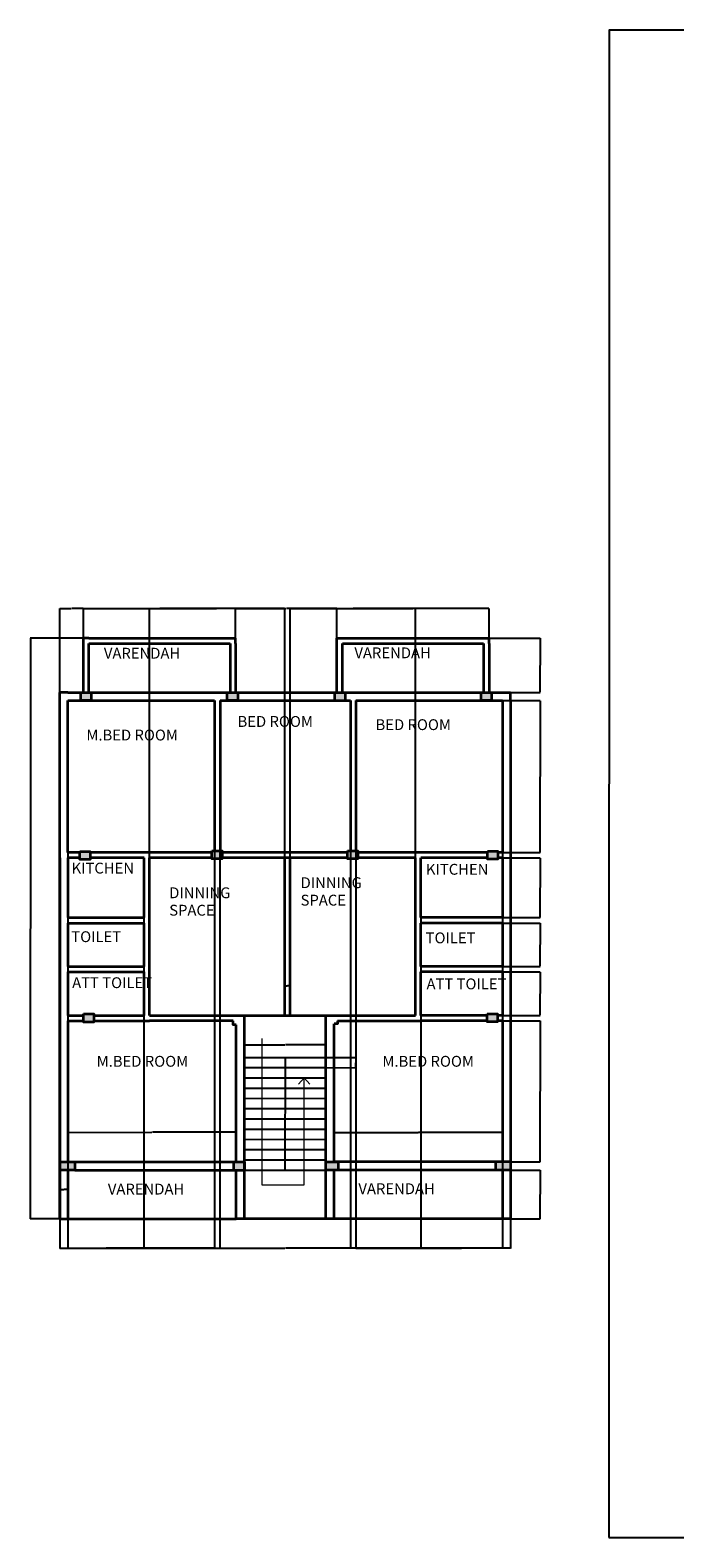
# Model space of a CAD drawing. Units: inches. Extents: x 328 to 2318, y 647 to 2548.
# Tile 1 of 5: x 328 to 1040, y 789 to 2456. Entities that reach past the tile are written whole.
import ezdxf

# ---------------------------------------------------------------- set-up
doc = ezdxf.new("R2010")
doc.units = ezdxf.units.IN
doc.header["$MEASUREMENT"] = 0
for name, color, linetype, lineweight in [('A-ANNO-DIMS', 2, 'Continuous', 18), ('A-ANNO-SYMB', 3, 'Continuous', 18), ('A-AREA-IDEN', 7, 'Continuous', 18), ('A-COLS', 1, 'Continuous', 35), ('A-FLOR-STRS', 7, 'Continuous', 25), ('A-WALL', 7, 'Continuous', 35)]:
    doc.layers.add(name, color=color, linetype=linetype, lineweight=lineweight)
doc.layers.add('A-COLS-PATT', color=18, linetype='Continuous', lineweight=13, true_color=0x000000)
doc.styles.get("Standard").update_dxf_attribs({"font": 'arial.ttf'})
doc.dimstyles.get("Standard").update_dxf_attribs({"dimtxt": 0.18, "dimasz": 0.18, "dimexe": 0.18, "dimexo": 0.0625, "dimgap": 0.09, "dimtad": 0, "dimtih": 1, "dimtoh": 1, "dimdec": 4, "dimzin": 0, "dimdsep": 46, "dimtxsty": 'Standard', "dimcen": 0.09, "dimadec": 0, "dimazin": 0, "dimtfac": 1, "dimtdec": 4, "dimtofl": 0, "dimtmove": 0, "dimatfit": 3, "dimfxl": 1, "dimtolj": 1, "dimtzin": 0, "dimarcsym": 0})

# ---------------------------------------------------------------- blocks, each defined once
blk = doc.blocks.new('*D13')
at = {"layer": 'A-ANNO-DIMS', "color": 0, "lineweight": -2, "transparency": 16777216}
for p, q in [((360.9, 1141.4), (360.9, 1108.7)), ((858.9, 1141.4), (858.9, 1108.7)), ((361.1, 1108.9), (609.7, 1108.9)), ((858.8, 1108.9), (610.2, 1108.9))]:
    blk.add_line(p, q, dxfattribs=at)
at = {"layer": 'A-ANNO-DIMS', "color": 0, "transparency": 16777216}
for points in [[(361.1, 1108.9), (361.1, 1108.8), (360.9, 1108.9)], [(858.8, 1108.9), (858.8, 1108.8), (858.9, 1108.9)]]:
    blk.add_solid(points, dxfattribs=at)
at = {"layer": 'Defpoints', "color": 0, "transparency": 16777216}
for p in [(360.9, 1141.4), (858.9, 1141.4), (858.9, 1108.9)]:
    blk.add_point(p, dxfattribs=at)
at = {"layer": 'A-ANNO-DIMS', "color": 0, "transparency": 16777216, "insert": (609.9, 1108.9), "char_height": 0.18, "attachment_point": 5}
blk.add_mtext('\\A1;498', dxfattribs=at)
blk = doc.blocks.new('*D14')
at = {"layer": 'A-ANNO-DIMS', "color": 0, "lineweight": -2, "transparency": 16777216}
for p, q in [((387, 1783.4), (328.2, 1783.4)), ((328.4, 1783.2), (328.4, 1462.6)), ((328.4, 1141.6), (328.4, 1462.2)), ((360.9, 1141.4), (328.2, 1141.4))]:
    blk.add_line(p, q, dxfattribs=at)
at = {"layer": 'A-ANNO-DIMS', "color": 0, "transparency": 16777216}
for points in [[(328.4, 1783.2), (328.4, 1783.2), (328.4, 1783.4)], [(328.4, 1141.6), (328.4, 1141.6), (328.4, 1141.4)]]:
    blk.add_solid(points, dxfattribs=at)
at = {"layer": 'Defpoints', "color": 0, "transparency": 16777216}
for p in [(328.4, 1783.4), (387, 1783.4), (360.9, 1141.4)]:
    blk.add_point(p, dxfattribs=at)
at = {"layer": 'A-ANNO-DIMS', "color": 0, "transparency": 16777216, "insert": (328.4, 1462.4), "char_height": 0.18, "attachment_point": 5}
blk.add_mtext('\\A1;642', dxfattribs=at)
blk = doc.blocks.new('*D15')
at = {"layer": 'A-ANNO-DIMS', "color": 0, "lineweight": -2, "transparency": 16777216}
for p, q in [((360.9, 1723.5), (360.9, 1816.2)), ((361.1, 1816), (373.5, 1816)), ((386.8, 1816), (374.4, 1816)), ((387, 1783.5), (387, 1816.2))]:
    blk.add_line(p, q, dxfattribs=at)
at = {"layer": 'A-ANNO-DIMS', "color": 0, "transparency": 16777216}
for points in [[(361.1, 1816), (361.1, 1815.9), (360.9, 1816)], [(386.8, 1816), (386.8, 1815.9), (387, 1816)]]:
    blk.add_solid(points, dxfattribs=at)
at = {"layer": 'Defpoints', "color": 0, "transparency": 16777216}
for p in [(387, 1816), (387, 1783.4), (360.9, 1723.4)]:
    blk.add_point(p, dxfattribs=at)
at = {"layer": 'A-ANNO-DIMS', "color": 0, "transparency": 16777216, "insert": (374, 1816), "char_height": 0.18, "attachment_point": 5}
blk.add_mtext('\\A1;26.067', dxfattribs=at)
blk = doc.blocks.new('*D16')
at = {"layer": 'A-ANNO-DIMS', "color": 0, "lineweight": -2, "transparency": 16777216}
for p, q in [((387, 1783.5), (387, 1816.2)), ((387.2, 1816), (470.7, 1816)), ((554.8, 1816), (471.3, 1816)), ((555, 1783.5), (555, 1816.2))]:
    blk.add_line(p, q, dxfattribs=at)
at = {"layer": 'A-ANNO-DIMS', "color": 0, "transparency": 16777216}
for points in [[(387.2, 1816), (387.2, 1815.9), (387, 1816)], [(554.8, 1816), (554.8, 1815.9), (555, 1816)]]:
    blk.add_solid(points, dxfattribs=at)
at = {"layer": 'Defpoints', "color": 0, "transparency": 16777216}
for p in [(555, 1816), (387, 1783.4), (555, 1783.4)]:
    blk.add_point(p, dxfattribs=at)
at = {"layer": 'A-ANNO-DIMS', "color": 0, "transparency": 16777216, "insert": (471, 1816), "char_height": 0.18, "attachment_point": 5}
blk.add_mtext('\\A1;168', dxfattribs=at)
blk = doc.blocks.new('*D17')
at = {"layer": 'A-ANNO-DIMS', "color": 0, "lineweight": -2, "transparency": 16777216}
for p, q in [((555, 1783.5), (555, 1816.2)), ((555.2, 1816), (610.6, 1816)), ((666.9, 1816), (611.5, 1816)), ((667.1, 1783.5), (667.1, 1816.2))]:
    blk.add_line(p, q, dxfattribs=at)
at = {"layer": 'A-ANNO-DIMS', "color": 0, "transparency": 16777216}
for points in [[(555.2, 1816), (555.2, 1815.9), (555, 1816)], [(666.9, 1816), (666.9, 1815.9), (667.1, 1816)]]:
    blk.add_solid(points, dxfattribs=at)
at = {"layer": 'Defpoints', "color": 0, "transparency": 16777216}
for p in [(667.1, 1816), (555, 1783.4), (667.1, 1783.4)]:
    blk.add_point(p, dxfattribs=at)
at = {"layer": 'A-ANNO-DIMS', "color": 0, "transparency": 16777216, "insert": (611.1, 1816), "char_height": 0.18, "attachment_point": 5}
blk.add_mtext('\\A1;112.09', dxfattribs=at)
blk = doc.blocks.new('*D18')
at = {"layer": 'A-ANNO-DIMS', "color": 0, "lineweight": -2, "transparency": 16777216}
for p, q in [((667.1, 1783.5), (667.1, 1816.2)), ((667.3, 1816), (750.8, 1816)), ((834.9, 1816), (751.4, 1816)), ((835.1, 1783.5), (835.1, 1816.2))]:
    blk.add_line(p, q, dxfattribs=at)
at = {"layer": 'A-ANNO-DIMS', "color": 0, "transparency": 16777216}
for points in [[(667.3, 1816), (667.3, 1815.9), (667.1, 1816)], [(834.9, 1816), (834.9, 1815.9), (835.1, 1816)]]:
    blk.add_solid(points, dxfattribs=at)
at = {"layer": 'Defpoints', "color": 0, "transparency": 16777216}
for p in [(835.1, 1816), (667.1, 1783.4), (835.1, 1783.4)]:
    blk.add_point(p, dxfattribs=at)
at = {"layer": 'A-ANNO-DIMS', "color": 0, "transparency": 16777216, "insert": (751.1, 1816), "char_height": 0.18, "attachment_point": 5}
blk.add_mtext('\\A1;168', dxfattribs=at)
blk = doc.blocks.new('*D19')
at = {"layer": 'A-ANNO-DIMS', "color": 0, "lineweight": -2, "transparency": 16777216}
for p, q in [((369.9, 1714.4), (369.9, 1108.7)), ((531.9, 1714.4), (531.9, 1108.7)), ((370.1, 1108.9), (450.7, 1108.9)), ((531.8, 1108.9), (451.2, 1108.9))]:
    blk.add_line(p, q, dxfattribs=at)
at = {"layer": 'A-ANNO-DIMS', "color": 0, "transparency": 16777216}
for points in [[(370.1, 1108.9), (370.1, 1108.8), (369.9, 1108.9)], [(531.8, 1108.9), (531.8, 1108.8), (531.9, 1108.9)]]:
    blk.add_solid(points, dxfattribs=at)
at = {"layer": 'Defpoints', "color": 0, "transparency": 16777216}
for p in [(369.9, 1714.4), (531.9, 1714.4), (531.9, 1108.9)]:
    blk.add_point(p, dxfattribs=at)
at = {"layer": 'A-ANNO-DIMS', "color": 0, "transparency": 16777216, "insert": (450.9, 1108.9), "char_height": 0.18, "attachment_point": 5}
blk.add_mtext('\\A1;162', dxfattribs=at)
blk = doc.blocks.new('*D20')
at = {"layer": 'A-ANNO-DIMS', "color": 0, "lineweight": -2, "transparency": 16777216}
for p, q in [((537.9, 1714.4), (537.9, 1108.7)), ((681.9, 1714.4), (681.9, 1108.7)), ((538.1, 1108.9), (609.7, 1108.9)), ((681.8, 1108.9), (610.2, 1108.9))]:
    blk.add_line(p, q, dxfattribs=at)
at = {"layer": 'A-ANNO-DIMS', "color": 0, "transparency": 16777216}
for points in [[(538.1, 1108.9), (538.1, 1108.8), (537.9, 1108.9)], [(681.8, 1108.9), (681.8, 1108.8), (681.9, 1108.9)]]:
    blk.add_solid(points, dxfattribs=at)
at = {"layer": 'Defpoints', "color": 0, "transparency": 16777216}
for p in [(537.9, 1714.4), (681.9, 1714.4), (681.9, 1108.9)]:
    blk.add_point(p, dxfattribs=at)
at = {"layer": 'A-ANNO-DIMS', "color": 0, "transparency": 16777216, "insert": (609.9, 1108.9), "char_height": 0.18, "attachment_point": 5}
blk.add_mtext('\\A1;144', dxfattribs=at)
blk = doc.blocks.new('*D21')
at = {"layer": 'A-ANNO-DIMS', "color": 0, "lineweight": -2, "transparency": 16777216}
for p, q in [((687.9, 1714.4), (687.9, 1108.7)), ((849.9, 1714.4), (849.9, 1108.7)), ((688.1, 1108.9), (768.7, 1108.9)), ((849.8, 1108.9), (769.2, 1108.9))]:
    blk.add_line(p, q, dxfattribs=at)
at = {"layer": 'A-ANNO-DIMS', "color": 0, "transparency": 16777216}
for points in [[(688.1, 1108.9), (688.1, 1108.8), (687.9, 1108.9)], [(849.8, 1108.9), (849.8, 1108.8), (849.9, 1108.9)]]:
    blk.add_solid(points, dxfattribs=at)
at = {"layer": 'Defpoints', "color": 0, "transparency": 16777216}
for p in [(687.9, 1714.4), (849.9, 1714.4), (849.9, 1108.9)]:
    blk.add_point(p, dxfattribs=at)
at = {"layer": 'A-ANNO-DIMS', "color": 0, "transparency": 16777216, "insert": (768.9, 1108.9), "char_height": 0.18, "attachment_point": 5}
blk.add_mtext('\\A1;162', dxfattribs=at)
blk = doc.blocks.new('*D22')
at = {"layer": 'A-ANNO-DIMS', "color": 0, "lineweight": -2, "transparency": 16777216}
for p, q in [((369.9, 1540.4), (369.9, 1108.7)), ((453.9, 1540.4), (453.9, 1108.7)), ((370.1, 1108.9), (411.7, 1108.9)), ((453.8, 1108.9), (412.2, 1108.9))]:
    blk.add_line(p, q, dxfattribs=at)
at = {"layer": 'A-ANNO-DIMS', "color": 0, "transparency": 16777216}
for points in [[(370.1, 1108.9), (370.1, 1108.8), (369.9, 1108.9)], [(453.8, 1108.9), (453.8, 1108.8), (453.9, 1108.9)]]:
    blk.add_solid(points, dxfattribs=at)
at = {"layer": 'Defpoints', "color": 0, "transparency": 16777216}
for p in [(369.9, 1540.4), (453.9, 1540.4), (453.9, 1108.9)]:
    blk.add_point(p, dxfattribs=at)
at = {"layer": 'A-ANNO-DIMS', "color": 0, "transparency": 16777216, "insert": (411.9, 1108.9), "char_height": 0.18, "attachment_point": 5}
blk.add_mtext('\\A1;84', dxfattribs=at)
blk = doc.blocks.new('*D23')
at = {"layer": 'A-ANNO-DIMS', "color": 0, "lineweight": -2, "transparency": 16777216}
for p, q in [((459.9, 1366.5), (459.9, 1816.2)), ((460.1, 1816), (534.2, 1816)), ((609.2, 1816), (535.1, 1816)), ((609.4, 1366.5), (609.4, 1816.2))]:
    blk.add_line(p, q, dxfattribs=at)
at = {"layer": 'A-ANNO-DIMS', "color": 0, "transparency": 16777216}
for points in [[(460.1, 1816), (460.1, 1815.9), (459.9, 1816)], [(609.2, 1816), (609.2, 1815.9), (609.4, 1816)]]:
    blk.add_solid(points, dxfattribs=at)
at = {"layer": 'Defpoints', "color": 0, "transparency": 16777216}
for p in [(609.4, 1816), (459.9, 1366.4), (609.4, 1366.4)]:
    blk.add_point(p, dxfattribs=at)
at = {"layer": 'A-ANNO-DIMS', "color": 0, "transparency": 16777216, "insert": (534.7, 1816), "char_height": 0.18, "attachment_point": 5}
blk.add_mtext('\\A1;149.44', dxfattribs=at)
blk = doc.blocks.new('*D24')
at = {"layer": 'A-ANNO-DIMS', "color": 0, "lineweight": -2, "transparency": 16777216}
for p, q in [((615.4, 1366.5), (615.4, 1816.2)), ((615.6, 1816), (684.2, 1816)), ((753.8, 1816), (685.1, 1816)), ((753.9, 1366.5), (753.9, 1816.2))]:
    blk.add_line(p, q, dxfattribs=at)
at = {"layer": 'A-ANNO-DIMS', "color": 0, "transparency": 16777216}
for points in [[(615.6, 1816), (615.6, 1815.9), (615.4, 1816)], [(753.8, 1816), (753.8, 1815.9), (753.9, 1816)]]:
    blk.add_solid(points, dxfattribs=at)
at = {"layer": 'Defpoints', "color": 0, "transparency": 16777216}
for p in [(753.9, 1816), (615.4, 1366.4), (753.9, 1366.4)]:
    blk.add_point(p, dxfattribs=at)
at = {"layer": 'A-ANNO-DIMS', "color": 0, "transparency": 16777216, "insert": (684.7, 1816), "char_height": 0.18, "attachment_point": 5}
blk.add_mtext('\\A1;138.56', dxfattribs=at)
blk = doc.blocks.new('*D25')
at = {"layer": 'A-ANNO-DIMS', "color": 0, "lineweight": -2, "transparency": 16777216}
for p, q in [((759.9, 1540.4), (759.9, 1108.7)), ((849.9, 1540.4), (849.9, 1108.7)), ((760.1, 1108.9), (804.7, 1108.9)), ((849.8, 1108.9), (805.2, 1108.9))]:
    blk.add_line(p, q, dxfattribs=at)
at = {"layer": 'A-ANNO-DIMS', "color": 0, "transparency": 16777216}
for points in [[(760.1, 1108.9), (760.1, 1108.8), (759.9, 1108.9)], [(849.8, 1108.9), (849.8, 1108.8), (849.9, 1108.9)]]:
    blk.add_solid(points, dxfattribs=at)
at = {"layer": 'Defpoints', "color": 0, "transparency": 16777216}
for p in [(759.9, 1540.4), (849.9, 1540.4), (849.9, 1108.9)]:
    blk.add_point(p, dxfattribs=at)
at = {"layer": 'A-ANNO-DIMS', "color": 0, "transparency": 16777216, "insert": (804.9, 1108.9), "char_height": 0.18, "attachment_point": 5}
blk.add_mtext('\\A1;90', dxfattribs=at)
blk = doc.blocks.new('*D26')
at = {"layer": 'A-ANNO-DIMS', "color": 0, "lineweight": -2, "transparency": 16777216}
for p, q in [((369.9, 1204.5), (369.9, 1237.2)), ((370.1, 1237), (462.6, 1237.1)), ((555.7, 1237.1), (463.2, 1237.1)), ((555.9, 1204.7), (555.9, 1237.3))]:
    blk.add_line(p, q, dxfattribs=at)
at = {"layer": 'A-ANNO-DIMS', "color": 0, "transparency": 16777216}
for points in [[(370.1, 1237), (370.1, 1236.9), (369.9, 1237)], [(555.7, 1237.2), (555.7, 1237.1), (555.9, 1237.1)]]:
    blk.add_solid(points, dxfattribs=at)
at = {"layer": 'Defpoints', "color": 0, "transparency": 16777216}
for p in [(555.9, 1237.1), (369.9, 1204.4), (555.9, 1204.6)]:
    blk.add_point(p, dxfattribs=at)
at = {"layer": 'A-ANNO-DIMS', "color": 0, "transparency": 16777216, "insert": (462.9, 1237.1), "char_height": 0.18, "attachment_point": 5}
blk.add_mtext('\\A1;186', dxfattribs=at)
blk = doc.blocks.new('*D27')
at = {"layer": 'A-ANNO-DIMS', "color": 0, "lineweight": -2, "transparency": 16777216}
for p, q in [((564.9, 1366.4), (564.9, 1333.7)), ((654.9, 1366.4), (654.9, 1333.7)), ((565.1, 1333.9), (609.7, 1333.9)), ((654.8, 1333.9), (610.2, 1333.9))]:
    blk.add_line(p, q, dxfattribs=at)
at = {"layer": 'A-ANNO-DIMS', "color": 0, "transparency": 16777216}
for points in [[(565.1, 1333.9), (565.1, 1333.8), (564.9, 1333.9)], [(654.8, 1333.9), (654.8, 1333.8), (654.9, 1333.9)]]:
    blk.add_solid(points, dxfattribs=at)
at = {"layer": 'Defpoints', "color": 0, "transparency": 16777216}
for p in [(564.9, 1366.4), (654.9, 1366.4), (564.9, 1333.9)]:
    blk.add_point(p, dxfattribs=at)
at = {"layer": 'A-ANNO-DIMS', "color": 0, "transparency": 16777216, "insert": (609.9, 1333.9), "char_height": 0.18, "attachment_point": 5}
blk.add_mtext('\\A1;90', dxfattribs=at)
blk = doc.blocks.new('*D28')
at = {"layer": 'A-ANNO-DIMS', "color": 0, "lineweight": -2, "transparency": 16777216}
for p, q in [((663.9, 1204.5), (663.9, 1237.2)), ((664.1, 1237), (756.7, 1237)), ((849.8, 1237), (757.2, 1237)), ((849.9, 1204.5), (849.9, 1237.2))]:
    blk.add_line(p, q, dxfattribs=at)
at = {"layer": 'A-ANNO-DIMS', "color": 0, "transparency": 16777216}
for points in [[(664.1, 1237), (664.1, 1236.9), (663.9, 1237)], [(849.8, 1237), (849.8, 1236.9), (849.9, 1237)]]:
    blk.add_solid(points, dxfattribs=at)
at = {"layer": 'Defpoints', "color": 0, "transparency": 16777216}
for p in [(849.9, 1237), (663.9, 1204.4), (849.9, 1204.4)]:
    blk.add_point(p, dxfattribs=at)
at = {"layer": 'A-ANNO-DIMS', "color": 0, "transparency": 16777216, "insert": (756.9, 1237), "char_height": 0.18, "attachment_point": 5}
blk.add_mtext('\\A1;186', dxfattribs=at)
blk = doc.blocks.new('*D29')
at = {"layer": 'A-ANNO-DIMS', "color": 0, "lineweight": -2, "transparency": 16777216}
for p, q in [((850, 1195.4), (891.7, 1195.4)), ((891.5, 1195.2), (891.5, 1168.6)), ((891.5, 1141.6), (891.5, 1168.2)), ((850, 1141.4), (891.7, 1141.4))]:
    blk.add_line(p, q, dxfattribs=at)
at = {"layer": 'A-ANNO-DIMS', "color": 0, "transparency": 16777216}
for points in [[(891.5, 1195.2), (891.5, 1195.2), (891.5, 1195.4)], [(891.5, 1141.6), (891.5, 1141.6), (891.5, 1141.4)]]:
    blk.add_solid(points, dxfattribs=at)
at = {"layer": 'Defpoints', "color": 0, "transparency": 16777216}
for p in [(849.9, 1195.4), (891.5, 1195.4), (849.9, 1141.4)]:
    blk.add_point(p, dxfattribs=at)
at = {"layer": 'A-ANNO-DIMS', "color": 0, "transparency": 16777216, "insert": (891.5, 1168.4), "char_height": 0.18, "attachment_point": 5}
blk.add_mtext('\\A1;54', dxfattribs=at)
blk = doc.blocks.new('*D30')
at = {"layer": 'A-ANNO-DIMS', "color": 0, "lineweight": -2, "transparency": 16777216}
for p, q in [((850, 1360.4), (891.7, 1360.4)), ((891.5, 1360.2), (891.5, 1282.6)), ((891.5, 1204.6), (891.5, 1282.2)), ((850, 1204.4), (891.7, 1204.4))]:
    blk.add_line(p, q, dxfattribs=at)
at = {"layer": 'A-ANNO-DIMS', "color": 0, "transparency": 16777216}
for points in [[(891.5, 1360.2), (891.5, 1360.2), (891.5, 1360.4)], [(891.5, 1204.6), (891.5, 1204.6), (891.5, 1204.4)]]:
    blk.add_solid(points, dxfattribs=at)
at = {"layer": 'Defpoints', "color": 0, "transparency": 16777216}
for p in [(849.9, 1360.4), (891.5, 1360.4), (849.9, 1204.4)]:
    blk.add_point(p, dxfattribs=at)
at = {"layer": 'A-ANNO-DIMS', "color": 0, "transparency": 16777216, "insert": (891.5, 1282.4), "char_height": 0.18, "attachment_point": 5}
blk.add_mtext('\\A1;156', dxfattribs=at)
blk = doc.blocks.new('*D31')
at = {"layer": 'A-ANNO-DIMS', "color": 0, "lineweight": -2, "transparency": 16777216}
for p, q in [((850, 1414.4), (891.7, 1414.4)), ((891.5, 1414.2), (891.5, 1390.6)), ((891.5, 1366.6), (891.5, 1390.2)), ((850, 1366.4), (891.7, 1366.4))]:
    blk.add_line(p, q, dxfattribs=at)
at = {"layer": 'A-ANNO-DIMS', "color": 0, "transparency": 16777216}
for points in [[(891.5, 1414.2), (891.5, 1414.2), (891.5, 1414.4)], [(891.5, 1366.6), (891.5, 1366.6), (891.5, 1366.4)]]:
    blk.add_solid(points, dxfattribs=at)
at = {"layer": 'Defpoints', "color": 0, "transparency": 16777216}
for p in [(849.9, 1414.4), (891.5, 1414.4), (849.9, 1366.4)]:
    blk.add_point(p, dxfattribs=at)
at = {"layer": 'A-ANNO-DIMS', "color": 0, "transparency": 16777216, "insert": (891.5, 1390.4), "char_height": 0.18, "attachment_point": 5}
blk.add_mtext('\\A1;48', dxfattribs=at)
blk = doc.blocks.new('*D32')
at = {"layer": 'A-ANNO-DIMS', "color": 0, "lineweight": -2, "transparency": 16777216}
for p, q in [((850, 1468.4), (891.7, 1468.4)), ((891.5, 1468.2), (891.5, 1444.6)), ((891.5, 1420.6), (891.5, 1444.2)), ((850, 1420.4), (891.7, 1420.4))]:
    blk.add_line(p, q, dxfattribs=at)
at = {"layer": 'A-ANNO-DIMS', "color": 0, "transparency": 16777216}
for points in [[(891.5, 1468.2), (891.5, 1468.2), (891.5, 1468.4)], [(891.5, 1420.6), (891.5, 1420.6), (891.5, 1420.4)]]:
    blk.add_solid(points, dxfattribs=at)
at = {"layer": 'Defpoints', "color": 0, "transparency": 16777216}
for p in [(849.9, 1468.4), (891.5, 1468.4), (849.9, 1420.4)]:
    blk.add_point(p, dxfattribs=at)
at = {"layer": 'A-ANNO-DIMS', "color": 0, "transparency": 16777216, "insert": (891.5, 1444.4), "char_height": 0.18, "attachment_point": 5}
blk.add_mtext('\\A1;48', dxfattribs=at)
blk = doc.blocks.new('*D33')
at = {"layer": 'A-ANNO-DIMS', "color": 0, "lineweight": -2, "transparency": 16777216}
for p, q in [((850, 1540.4), (891.7, 1540.4)), ((891.5, 1540.2), (891.5, 1507.6)), ((891.5, 1474.6), (891.5, 1507.2)), ((850, 1474.4), (891.7, 1474.4))]:
    blk.add_line(p, q, dxfattribs=at)
at = {"layer": 'A-ANNO-DIMS', "color": 0, "transparency": 16777216}
for points in [[(891.5, 1540.2), (891.5, 1540.2), (891.5, 1540.4)], [(891.5, 1474.6), (891.5, 1474.6), (891.5, 1474.4)]]:
    blk.add_solid(points, dxfattribs=at)
at = {"layer": 'Defpoints', "color": 0, "transparency": 16777216}
for p in [(849.9, 1540.4), (891.5, 1540.4), (849.9, 1474.4)]:
    blk.add_point(p, dxfattribs=at)
at = {"layer": 'A-ANNO-DIMS', "color": 0, "transparency": 16777216, "insert": (891.5, 1507.4), "char_height": 0.18, "attachment_point": 5}
blk.add_mtext('\\A1;66', dxfattribs=at)
blk = doc.blocks.new('*D34')
at = {"layer": 'A-ANNO-DIMS', "color": 0, "lineweight": -2, "transparency": 16777216}
for p, q in [((850, 1714.4), (891.7, 1714.4)), ((891.5, 1714.2), (891.5, 1630.6)), ((891.5, 1546.6), (891.5, 1630.2)), ((850, 1546.4), (891.7, 1546.4))]:
    blk.add_line(p, q, dxfattribs=at)
at = {"layer": 'A-ANNO-DIMS', "color": 0, "transparency": 16777216}
for points in [[(891.5, 1714.2), (891.5, 1714.2), (891.5, 1714.4)], [(891.5, 1546.6), (891.5, 1546.6), (891.5, 1546.4)]]:
    blk.add_solid(points, dxfattribs=at)
at = {"layer": 'Defpoints', "color": 0, "transparency": 16777216}
for p in [(849.9, 1714.4), (891.5, 1714.4), (849.9, 1546.4)]:
    blk.add_point(p, dxfattribs=at)
at = {"layer": 'A-ANNO-DIMS', "color": 0, "transparency": 16777216, "insert": (891.5, 1630.4), "char_height": 0.18, "attachment_point": 5}
blk.add_mtext('\\A1;168', dxfattribs=at)
blk = doc.blocks.new('*D35')
at = {"layer": 'A-ANNO-DIMS', "color": 0, "lineweight": -2, "transparency": 16777216}
for p, q in [((835.2, 1783.4), (891.7, 1783.4)), ((891.5, 1783.2), (891.5, 1753.6)), ((891.5, 1723.6), (891.5, 1753.2)), ((835.2, 1723.4), (891.7, 1723.4))]:
    blk.add_line(p, q, dxfattribs=at)
at = {"layer": 'A-ANNO-DIMS', "color": 0, "transparency": 16777216}
for points in [[(891.5, 1783.2), (891.5, 1783.2), (891.5, 1783.4)], [(891.5, 1723.6), (891.5, 1723.6), (891.5, 1723.4)]]:
    blk.add_solid(points, dxfattribs=at)
at = {"layer": 'Defpoints', "color": 0, "transparency": 16777216}
for p in [(835.1, 1783.4), (891.5, 1783.4), (835.1, 1723.4)]:
    blk.add_point(p, dxfattribs=at)
at = {"layer": 'A-ANNO-DIMS', "color": 0, "transparency": 16777216, "insert": (891.5, 1753.4), "char_height": 0.18, "attachment_point": 5}
blk.add_mtext('\\A1;60', dxfattribs=at)
blk = doc.blocks.new('*D36')
at = {"layer": 'A-ANNO-DIMS', "color": 0, "lineweight": -2, "transparency": 16777216}
for p, q in [((360.9, 1141.5), (360.9, 1174.2)), ((361.1, 1174), (365.3, 1174)), ((369.8, 1174), (365.6, 1174)), ((369.9, 1141.5), (369.9, 1174.2))]:
    blk.add_line(p, q, dxfattribs=at)
at = {"layer": 'A-ANNO-DIMS', "color": 0, "transparency": 16777216}
for points in [[(361.1, 1174), (361.1, 1173.9), (360.9, 1174)], [(369.8, 1174), (369.8, 1173.9), (369.9, 1174)]]:
    blk.add_solid(points, dxfattribs=at)
at = {"layer": 'Defpoints', "color": 0, "transparency": 16777216}
for p in [(369.9, 1174), (360.9, 1141.4), (369.9, 1141.4)]:
    blk.add_point(p, dxfattribs=at)
at = {"layer": 'A-ANNO-DIMS', "color": 0, "transparency": 16777216, "insert": (365.4, 1174), "char_height": 0.18, "attachment_point": 5}
blk.add_mtext('\\A1;9', dxfattribs=at)
blk = doc.blocks.new('*D37')
at = {"layer": 'A-ANNO-DIMS', "color": 0, "lineweight": -2, "transparency": 16777216}
for p, q in [((609.4, 1366.5), (609.4, 1399.2)), ((609.6, 1399), (612.2, 1399)), ((615.2, 1399), (612.5, 1399)), ((615.4, 1366.5), (615.4, 1399.2))]:
    blk.add_line(p, q, dxfattribs=at)
at = {"layer": 'A-ANNO-DIMS', "color": 0, "transparency": 16777216}
for points in [[(609.6, 1399), (609.6, 1398.9), (609.4, 1399)], [(615.2, 1399), (615.2, 1398.9), (615.4, 1399)]]:
    blk.add_solid(points, dxfattribs=at)
at = {"layer": 'Defpoints', "color": 0, "transparency": 16777216}
for p in [(615.4, 1399), (609.4, 1366.4), (615.4, 1366.4)]:
    blk.add_point(p, dxfattribs=at)
at = {"layer": 'A-ANNO-DIMS', "color": 0, "transparency": 16777216, "insert": (612.4, 1399), "char_height": 0.18, "attachment_point": 5}
blk.add_mtext('\\A1;6', dxfattribs=at)
blk = doc.blocks.new('*D38')
at = {"layer": 'A-ANNO-DIMS', "color": 0, "lineweight": -2, "transparency": 16777216}
for p, q in [((655.4, 1319.9), (688.1, 1319.8)), ((687.9, 1319.6), (687.9, 1314.3)), ((655.3, 1308.6), (688, 1308.5)), ((687.8, 1308.7), (687.9, 1314))]:
    blk.add_line(p, q, dxfattribs=at)
at = {"layer": 'A-ANNO-DIMS', "color": 0, "transparency": 16777216}
for points in [[(687.8, 1319.6), (687.9, 1319.6), (687.9, 1319.8)], [(687.8, 1308.7), (687.9, 1308.7), (687.8, 1308.5)]]:
    blk.add_solid(points, dxfattribs=at)
at = {"layer": 'Defpoints', "color": 0, "transparency": 16777216}
for p in [(655.3, 1319.9), (655.3, 1308.6), (687.8, 1308.5)]:
    blk.add_point(p, dxfattribs=at)
at = {"layer": 'A-ANNO-DIMS', "color": 0, "transparency": 16777216, "insert": (687.9, 1314.2), "char_height": 0.18, "attachment_point": 5}
blk.add_mtext('\\A1;11.323', dxfattribs=at)
blk = doc.blocks.new('*D40')
at = {"layer": 'A-ANNO-DIMS', "color": 0, "lineweight": -2, "transparency": 16777216}
for p, q in [((1362.3, 2455.5), (967.6, 2455.5)), ((967.8, 2455.4), (967.8, 1622.3)), ((967.8, 789), (967.8, 1622)), ((1076.4, 788.8), (967.6, 788.8))]:
    blk.add_line(p, q, dxfattribs=at)
at = {"layer": 'A-ANNO-DIMS', "color": 0, "transparency": 16777216}
for points in [[(967.8, 2455.4), (967.9, 2455.4), (967.8, 2455.5)], [(967.8, 789), (967.9, 789), (967.8, 788.8)]]:
    blk.add_solid(points, dxfattribs=at)
at = {"layer": 'Defpoints', "color": 0, "transparency": 16777216}
for p in [(967.8, 2455.5), (1362.4, 2455.5), (1076.4, 788.8)]:
    blk.add_point(p, dxfattribs=at)
at = {"layer": 'A-ANNO-DIMS', "color": 0, "transparency": 16777216, "insert": (967.8, 1622.2), "char_height": 0.18, "attachment_point": 5}
blk.add_mtext('\\A1;1666.7', dxfattribs=at)

msp = doc.modelspace()

# ---------------------------------------------------------------- hatches: boundary and pattern name
at = {"layer": 'A-COLS-PATT'}
h = msp.add_hatch(color=256, dxfattribs=at)
h.dxf.hatch_style = 1
h.paths.add_polyline_path([(377.3633, 1204.4262), (360.9477, 1204.4262), (360.9477, 1195.2087), (377.3633, 1195.2087)])
h.paths.add_polyline_path([(398.5016, 1367.9244), (387.0471, 1367.9244), (387.0471, 1358.9244), (398.5016, 1358.9244)])
h.paths.add_polyline_path([(844.6513, 1368.1659), (833.1969, 1368.1659), (833.1969, 1359.1659), (844.6513, 1359.1659)])
h.paths.add_polyline_path([(844.856, 1548.0886), (833.4015, 1548.0886), (833.4015, 1539.0886), (844.856, 1539.0886)])
h.paths.add_polyline_path([(690.1724, 1548.4286), (678.718, 1548.4286), (678.718, 1539.4286), (690.1724, 1539.4286)])
h.paths.add_polyline_path([(540.2842, 1548.3838), (528.8297, 1548.3838), (528.8297, 1539.3838), (540.2842, 1539.3838)])
h.paths.add_polyline_path([(394.383, 1547.6165), (382.9285, 1547.6165), (382.9285, 1538.6165), (394.383, 1538.6165)])
h.paths.add_polyline_path([(395.6596, 1723.4262), (384.2051, 1723.4262), (384.2051, 1714.4262), (395.6596, 1714.4262)])
h.paths.add_polyline_path([(557.4545, 1723.4262), (546.0001, 1723.4262), (546.0001, 1714.4262), (557.4545, 1714.4262)])
h.paths.add_polyline_path([(676.224, 1723.4262), (667.1032, 1723.4262), (664.7696, 1723.4262), (664.7696, 1714.4262), (676.224, 1714.4262)])
h.paths.add_polyline_path([(837.9857, 1723.4262), (835.1032, 1723.4262), (829.1032, 1723.4292), (829.1032, 1723.4262), (826.5312, 1723.4262), (826.5312, 1714.4305), (837.9857, 1714.4305)])
h.paths.add_polyline_path([(564.9477, 1204.5884), (553.1198, 1204.5884), (553.1198, 1195.4262), (564.9477, 1195.4262)])
h.paths.add_polyline_path([(668.5315, 1204.3548), (654.9477, 1204.3548), (654.9477, 1195.3548), (663.9477, 1195.3548), (663.9477, 1195.4262), (668.5315, 1195.4262)])
h.paths.add_polyline_path([(858.9477, 1204.4262), (842.7029, 1204.4262), (842.7029, 1195.4262), (858.9477, 1195.4262)])

# ---------------------------------------------------------------- linework, layer by layer
at = {"layer": 'A-ANNO-SYMB'}
for p, q in [((584.175, 1340.7847), (584.175, 1179.1207)), ((630.9349, 1297.2849), (624.5503, 1290.3905)), ((630.8416, 1179.1207), (630.9349, 1297.2849)), ((630.9349, 1297.2849), (637.3086, 1290.3805)), ((584.175, 1179.1207), (630.8416, 1179.1207))]:
    msp.add_line(p, q, dxfattribs=at)
at = {"layer": 'A-COLS'}
msp.add_line((553.1198, 1195.4262), (564.5743, 1195.4262), dxfattribs=at)
for points in [[(384.2051, 1723.4262), (395.6596, 1723.4262), (395.6596, 1714.4262), (384.2051, 1714.4262)], [(546.0001, 1723.4262), (557.4545, 1723.4262), (557.4545, 1714.4262), (546.0001, 1714.4262)], [(826.5312, 1723.4305), (837.9857, 1723.4305), (837.9857, 1714.4305), (826.5312, 1714.4305)], [(382.9285, 1547.6165), (394.383, 1547.6165), (394.383, 1538.6165), (382.9285, 1538.6165)], [(528.8297, 1548.3838), (540.2842, 1548.3838), (540.2842, 1539.3838), (528.8297, 1539.3838)], [(678.718, 1548.4286), (690.1724, 1548.4286), (690.1724, 1539.4286), (678.718, 1539.4286)], [(833.4015, 1548.0886), (844.856, 1548.0886), (844.856, 1539.0886), (833.4015, 1539.0886)], [(387.0471, 1367.9244), (398.5016, 1367.9244), (398.5016, 1358.9244), (387.0471, 1358.9244)], [(833.1969, 1368.1659), (844.6513, 1368.1659), (844.6513, 1359.1659), (833.1969, 1359.1659)], [(654.9477, 1204.3548), (668.5315, 1204.3548), (668.5315, 1195.3548), (654.9477, 1195.3548)]]:
    msp.add_lwpolyline(points, close=True, dxfattribs=at)
for points in [[(664.7696, 1714.5103), (664.7696, 1723.4262)], [(676.224, 1723.4262), (676.224, 1714.5103)], [(377.3633, 1204.4262), (377.3633, 1195.2087), (360.9477, 1195.2087), (360.9477, 1204.4262)], [(553.1198, 1195.4262), (553.1198, 1204.5884), (564.9477, 1204.5884), (564.9477, 1195.4262)], [(858.9477, 1195.4262), (842.7029, 1195.4262), (842.7029, 1204.4262)]]:
    msp.add_lwpolyline(points, dxfattribs=at)
at = {"layer": 'A-FLOR-STRS'}
for p, q in [((564.9477, 1319.9838), (655.321, 1319.9125)), ((609.761, 1195.3905), (610.1344, 1319.9482)), ((564.9137, 1308.6604), (655.2871, 1308.5891)), ((564.8458, 1286.0136), (655.2192, 1285.9422)), ((564.8798, 1297.337), (655.2532, 1297.2657)), ((564.8119, 1274.6901), (655.1853, 1274.6188)), ((564.744, 1252.0433), (655.1174, 1251.972)), ((564.7779, 1263.3667), (655.1513, 1263.2954)), ((564.71, 1240.7199), (655.0834, 1240.6485)), ((564.6422, 1218.073), (655.0155, 1218.0017)), ((564.6761, 1229.3964), (655.0495, 1229.3251)), ((564.6082, 1206.7496), (654.9816, 1206.6782)), ((564.5743, 1195.4262), (654.9477, 1195.3548))]:
    msp.add_line(p, q, dxfattribs=at)
at = {"layer": 'A-WALL'}
for p, q in [((393.0144, 1783.4262), (387.0144, 1783.4262)), ((387.0144, 1777.4262), (387.0144, 1783.4262)), ((393.0144, 1783.4262), (549.0144, 1783.4262)), ((549.0144, 1783.4262), (555.0144, 1783.4262)), ((555.0144, 1777.4262), (555.0144, 1783.4262)), ((667.1032, 1783.4262), (835.1032, 1783.4262)), ((667.1032, 1777.4262), (667.1032, 1783.4262)), ((835.1032, 1777.4262), (835.1032, 1783.4262)), ((387.0144, 1723.4262), (387.0144, 1777.4262)), ((393.0144, 1723.4262), (393.0144, 1777.4262)), ((393.0144, 1777.4262), (549.0144, 1777.4262)), ((549.0144, 1777.4262), (549.0144, 1723.4262)), ((555.0144, 1777.4262), (555.0144, 1723.4262)), ((667.1032, 1723.4262), (667.1032, 1777.4262)), ((673.1032, 1723.4262), (673.1032, 1777.4262)), ((673.1032, 1777.4262), (829.1032, 1777.4262)), ((829.1032, 1777.4262), (829.1032, 1723.4262)), ((835.1032, 1777.4262), (835.1032, 1723.4262)), ((369.9477, 1723.4262), (360.9477, 1723.4262)), ((360.9477, 1714.4262), (360.9477, 1723.4262)), ((369.9477, 1723.4262), (387.0144, 1723.4262)), ((393.0144, 1723.4262), (549.0144, 1723.4262)), ((555.0144, 1723.4262), (667.1032, 1723.4262)), ((667.1032, 1723.4262), (829.1032, 1723.4262)), ((835.1032, 1723.4262), (849.9477, 1723.4262)), ((849.9477, 1723.4262), (858.9477, 1723.4262)), ((858.9477, 1714.4262), (858.9477, 1723.4262)), ((360.9477, 1141.4262), (360.9477, 1714.4262)), ((369.9477, 1714.4262), (531.9477, 1714.4262)), ((369.9477, 1546.4262), (369.9477, 1714.4262)), ((531.9477, 1714.4262), (531.9477, 1548.3838)), ((537.9477, 1714.4262), (537.9477, 1548.3838)), ((537.9477, 1714.4262), (681.9477, 1714.4262)), ((681.9477, 1714.4262), (681.9477, 1548.4286)), ((687.9477, 1714.4262), (687.9477, 1548.4286)), ((687.9477, 1714.4262), (849.9477, 1714.4262)), ((849.9477, 1714.4262), (849.9477, 1546.4262)), ((858.9477, 1714.4262), (858.9477, 1546.4262)), ((360.9477, 1540.4262), (360.9477, 1141.4262)), ((382.9285, 1546.4262), (369.9477, 1546.4262)), ((369.9477, 1540.4262), (369.9477, 1474.4262)), ((382.9285, 1540.4262), (369.9477, 1540.4262)), ((528.8297, 1546.4262), (394.383, 1546.4262)), ((453.9477, 1540.4262), (394.383, 1540.4262)), ((453.9477, 1474.4262), (453.9477, 1540.4262)), ((528.8297, 1540.4262), (459.9477, 1540.4262)), ((459.9477, 1474.4262), (459.9477, 1540.4262)), ((528.8297, 1540.4262), (459.9477, 1540.4262)), ((678.718, 1546.4262), (540.2842, 1546.4262)), ((678.718, 1540.4262), (540.2842, 1540.4262)), ((678.718, 1540.4262), (540.2842, 1540.4262)), ((609.3887, 1366.4262), (609.3887, 1540.4262)), ((615.3887, 1366.4262), (615.3887, 1540.4262)), ((833.4015, 1546.4262), (690.1724, 1546.4262)), ((753.9477, 1540.4262), (690.1724, 1540.4262)), ((753.9477, 1366.4262), (753.9477, 1540.4262)), ((753.9477, 1474.4262), (753.9477, 1540.4262)), ((759.9477, 1474.4262), (759.9477, 1540.4262)), ((833.4015, 1540.4262), (759.9477, 1540.4262)), ((849.9477, 1546.4262), (844.856, 1546.4262)), ((849.9477, 1540.4262), (844.856, 1540.4262)), ((849.9477, 1540.4262), (849.9477, 1474.4262)), ((858.9477, 1546.4262), (858.9477, 1540.4262)), ((858.9477, 1540.4262), (858.9477, 1141.4262)), ((360.9477, 1468.4262), (360.9477, 1141.4262)), ((369.9477, 1474.4262), (453.9477, 1474.4262)), ((369.9477, 1468.4262), (453.9477, 1468.4262)), ((369.9477, 1468.4262), (369.9477, 1420.4262)), ((453.9477, 1420.4262), (453.9477, 1468.4262)), ((459.9477, 1414.4262), (459.9477, 1474.4262)), ((753.9477, 1420.4262), (753.9477, 1468.4262)), ((849.9477, 1474.4262), (759.9477, 1474.4262)), ((849.9477, 1468.4262), (759.9477, 1468.4262)), ((759.9477, 1420.4262), (759.9477, 1468.4262)), ((849.9477, 1468.4262), (849.9477, 1420.4262)), ((858.9477, 1468.4262), (858.9477, 1141.4262)), ((369.9477, 1420.4262), (453.9477, 1420.4262)), ((849.9477, 1420.4262), (759.9477, 1420.4262)), ((360.9477, 1414.4262), (360.9477, 1141.4262)), ((369.9477, 1414.4262), (453.9477, 1414.4262)), ((369.9477, 1414.4262), (369.9477, 1366.4262)), ((453.9477, 1366.4262), (453.9477, 1414.4262)), ((459.9477, 1366.4262), (459.9477, 1414.4262)), ((849.9477, 1414.4262), (759.9477, 1414.4262)), ((759.9477, 1366.4262), (759.9477, 1414.4262)), ((849.9477, 1414.4262), (849.9477, 1366.4262)), ((858.9477, 1414.4262), (858.9477, 1141.4262)), ((360.9477, 1360.4262), (360.9477, 1141.4262)), ((369.9477, 1366.4262), (387.0471, 1366.4262)), ((369.9477, 1360.4262), (387.0471, 1360.4262)), ((369.9477, 1360.4262), (369.9477, 1204.4262)), ((398.5016, 1366.4262), (453.9477, 1366.4262)), ((398.5016, 1360.4262), (459.9477, 1360.4262)), ((459.9477, 1366.4262), (654.9477, 1366.4262)), ((552.4018, 1360.4262), (459.9477, 1360.4262)), ((555.9477, 1204.5884), (555.9477, 1355.8275)), ((564.9477, 1141.4262), (564.9477, 1366.4262)), ((654.9477, 1141.4262), (654.9477, 1366.4262)), ((654.9477, 1366.4262), (753.9477, 1366.4262)), ((663.9477, 1204.4262), (663.9477, 1357.1438)), ((667.8862, 1360.4262), (759.9477, 1360.4262)), ((833.1969, 1366.4262), (759.9477, 1366.4262)), ((833.1969, 1360.4262), (759.9477, 1360.4262)), ((849.9477, 1366.4262), (844.6513, 1366.4262)), ((849.9477, 1360.4262), (844.6513, 1360.4262)), ((849.9477, 1360.4262), (849.9477, 1204.4262)), ((858.9477, 1360.4262), (858.9477, 1141.4262)), ((360.9477, 1204.4262), (553.1198, 1204.4262)), ((858.9477, 1204.4262), (663.9477, 1204.4262)), ((360.9477, 1195.4262), (360.9477, 1141.4262)), ((369.9477, 1195.2087), (369.9477, 1141.4262)), ((377.3633, 1195.4262), (555.9477, 1195.4262)), ((555.9477, 1141.4262), (555.9477, 1195.4262)), ((849.9477, 1195.4262), (663.9477, 1195.4262)), ((663.9477, 1141.4262), (663.9477, 1195.4262)), ((849.9477, 1195.4262), (849.9477, 1141.4262)), ((858.9477, 1195.4262), (858.9477, 1141.4262)), ((360.9477, 1141.4262), (555.9477, 1141.4262)), ((858.9477, 1141.4262), (555.9477, 1141.4262))]:
    msp.add_line(p, q, dxfattribs=at)
for points in [[(555.9477, 1355.8275), (552.4018, 1355.8275), (552.4018, 1360.4262)], [(667.8862, 1360.4262), (667.8862, 1357.1438), (663.9477, 1357.1438)]]:
    msp.add_lwpolyline(points, dxfattribs=at)

# ---------------------------------------------------------------- texts
at = {"layer": 'A-AREA-IDEN'}
for s, p in [('VARENDAH', (409.6343, 1760.7557)), ('VARENDAH', (686.4131, 1761.1502)), ('BED ROOM', (557.2761, 1685.2946)), ('BED ROOM', (709.7481, 1681.7695)), ('M.BED ROOM', (390.2776, 1670.2702)), ('KITCHEN', (373.9399, 1523.1669)), ('KITCHEN', (765.4248, 1521.8694)), ('DINNING ', (626.941, 1507.0382)), ('DINNING', (481.7976, 1495.8952)), ('SPACE', (481.7976, 1476.6183)), ('SPACE', (626.941, 1487.7613)), ('TOILET', (373.6347, 1447.3575)), ('TOILET', (765.1196, 1446.06)), ('ATT TOILET', (374.5633, 1396.4935)), ('ATT TOILET', (766.0482, 1395.196)), ('M.BED ROOM', (401.649, 1309.6058)), ('M.BED ROOM', (717.3335, 1309.6058)), ('VARENDAH', (414.0377, 1168.3256)), ('VARENDAH', (690.8164, 1168.7201))]:
    msp.add_text(s, height=12, dxfattribs=at).set_placement(p)

# ---------------------------------------------------------------- dimensions: what is measured, and where the dimension line sits
at = {"layer": 'A-ANNO-DIMS'}
for base, p1, p2, angle, override, picture, middle in [((967.826, 2455.5387), (1076.4266, 788.791), (1362.3871, 2455.5387), 90, {"dimdec": 1, "dimlfac": 1, "dimrnd": 0, "dimzin": 0, "dimdsep": 46, "dimlunit": 2}, '*D40', (967.826, 1622.1648)), ((328.3977, 1783.4262), (360.9477, 1141.4262), (387.0144, 1783.4262), 90, {"dimdec": 0, "dimlfac": 1, "dimrnd": 0, "dimzin": 0, "dimdsep": 46, "dimlunit": 2}, '*D14', (328.3977, 1462.4262)), ((891.4977, 1783.4262), (835.1032, 1723.4262), (835.1032, 1783.4262), 90, {"dimdec": 0, "dimlfac": 1, "dimrnd": 0, "dimzin": 0, "dimdsep": 46, "dimlunit": 2}, '*D35', (891.4977, 1753.4262)), ((891.4977, 1714.4262), (849.9477, 1546.4262), (849.9477, 1714.4262), 90, {"dimdec": 0, "dimlfac": 1, "dimrnd": 0, "dimzin": 0, "dimdsep": 46, "dimlunit": 2}, '*D34', (891.4977, 1630.4262)), ((891.4977, 1540.4262), (849.9477, 1474.4262), (849.9477, 1540.4262), 90, {"dimdec": 0, "dimlfac": 1, "dimrnd": 0, "dimzin": 0, "dimdsep": 46, "dimlunit": 2}, '*D33', (891.4977, 1507.4262)), ((891.4977, 1468.4262), (849.9477, 1420.4262), (849.9477, 1468.4262), 90, {"dimdec": 0, "dimlfac": 1, "dimrnd": 0, "dimzin": 0, "dimdsep": 46, "dimlunit": 2}, '*D32', (891.4977, 1444.4262)), ((891.4977, 1414.4262), (849.9477, 1366.4262), (849.9477, 1414.4262), 90, {"dimdec": 0, "dimlfac": 1, "dimrnd": 0, "dimzin": 0, "dimdsep": 46, "dimlunit": 2}, '*D31', (891.4977, 1390.4262)), ((564.9477, 1333.8762), (654.9477, 1366.4262), (564.9477, 1366.4262), 180, {"dimdec": 0, "dimlfac": 1, "dimrnd": 0, "dimzin": 0, "dimdsep": 46, "dimlunit": 2}, '*D27', (609.9477, 1333.8762)), ((891.4977, 1360.4262), (849.9477, 1204.4262), (849.9477, 1360.4262), 90, {"dimdec": 0, "dimlfac": 1, "dimrnd": 0, "dimzin": 0, "dimdsep": 46, "dimlunit": 2}, '*D30', (891.4977, 1282.4262)), ((687.837, 1308.4915), (655.321, 1319.9125), (655.2871, 1308.5891), 269.828245, {"dimdec": 3, "dimlfac": 1, "dimrnd": 0, "dimzin": 0, "dimdsep": 46, "dimlunit": 2}, '*D38', (687.8539, 1314.1532)), ((555.9193, 1237.1384), (369.9477, 1204.4262), (555.9477, 1204.5884), 0.0499907, {"dimdec": 0, "dimlfac": 1, "dimrnd": 0, "dimzin": 0, "dimdsep": 46, "dimlunit": 2}, '*D26', (462.9193, 1237.0573)), ((891.4977, 1195.4262), (849.9477, 1141.4262), (849.9477, 1195.4262), 90, {"dimdec": 0, "dimlfac": 1, "dimrnd": 0, "dimzin": 0, "dimdsep": 46, "dimlunit": 2}, '*D29', (891.4977, 1168.4262))]:
    dim = msp.add_linear_dim(base=base, p1=p1, p2=p2, angle=angle, dimstyle='Standard', override=override, dxfattribs=at)
    dim.commit()
    dim.dimension.update_dxf_attribs({"geometry": picture, "text_midpoint": middle})
for base, p1, p2, override, picture, middle in [((387.0144, 1815.9761), (360.9477, 1723.4262), (387.0144, 1783.4262), {"dimdec": 3, "dimlfac": 1, "dimrnd": 0, "dimzin": 0, "dimdsep": 46, "dimlunit": 2}, '*D15', (373.9811, 1815.9761)), ((555.0144, 1815.9761), (387.0144, 1783.4262), (555.0144, 1783.4262), {"dimdec": 0, "dimlfac": 1, "dimrnd": 0, "dimzin": 0, "dimdsep": 46, "dimlunit": 2}, '*D16', (471.0144, 1815.9761)), ((609.3887, 1815.9761), (459.9477, 1366.4262), (609.3887, 1366.4262), {"dimdec": 2, "dimlfac": 1, "dimrnd": 0, "dimzin": 0, "dimdsep": 46, "dimlunit": 2}, '*D23', (534.6682, 1815.9761)), ((667.1032, 1815.9761), (555.0144, 1783.4262), (667.1032, 1783.4262), {"dimdec": 2, "dimlfac": 1, "dimrnd": 0, "dimzin": 0, "dimdsep": 46, "dimlunit": 2}, '*D17', (611.0588, 1815.9761)), ((753.9477, 1815.9761), (615.3887, 1366.4262), (753.9477, 1366.4262), {"dimdec": 2, "dimlfac": 1, "dimrnd": 0, "dimzin": 0, "dimdsep": 46, "dimlunit": 2}, '*D24', (684.6682, 1815.9761)), ((835.1032, 1815.9761), (667.1032, 1783.4262), (835.1032, 1783.4262), {"dimdec": 0, "dimlfac": 1, "dimrnd": 0, "dimzin": 0, "dimdsep": 46, "dimlunit": 2}, '*D18', (751.1032, 1815.9761)), ((531.9477, 1108.8762), (369.9477, 1714.4262), (531.9477, 1714.4262), {"dimdec": 0, "dimlfac": 1, "dimrnd": 0, "dimzin": 0, "dimdsep": 46, "dimlunit": 2}, '*D19', (450.9477, 1108.8762)), ((681.9477, 1108.8762), (537.9477, 1714.4262), (681.9477, 1714.4262), {"dimdec": 0, "dimlfac": 1, "dimrnd": 0, "dimzin": 0, "dimdsep": 46, "dimlunit": 2}, '*D20', (609.9477, 1108.8762)), ((849.9477, 1108.8762), (687.9477, 1714.4262), (849.9477, 1714.4262), {"dimdec": 0, "dimlfac": 1, "dimrnd": 0, "dimzin": 0, "dimdsep": 46, "dimlunit": 2}, '*D21', (768.9477, 1108.8762)), ((453.9477, 1108.8762), (369.9477, 1540.4262), (453.9477, 1540.4262), {"dimdec": 0, "dimlfac": 1, "dimrnd": 0, "dimzin": 0, "dimdsep": 46, "dimlunit": 2}, '*D22', (411.9477, 1108.8762)), ((849.9477, 1108.8762), (759.9477, 1540.4262), (849.9477, 1540.4262), {"dimdec": 0, "dimlfac": 1, "dimrnd": 0, "dimzin": 0, "dimdsep": 46, "dimlunit": 2}, '*D25', (804.9477, 1108.8762)), ((615.3887, 1398.9761), (609.3887, 1366.4262), (615.3887, 1366.4262), {"dimdec": 0, "dimlfac": 1, "dimrnd": 0, "dimzin": 0, "dimdsep": 46, "dimlunit": 2}, '*D37', (612.3887, 1398.9761)), ((849.9477, 1236.9761), (663.9477, 1204.4262), (849.9477, 1204.4262), {"dimdec": 0, "dimlfac": 1, "dimrnd": 0, "dimzin": 0, "dimdsep": 46, "dimlunit": 2}, '*D28', (756.9477, 1236.9761)), ((369.9477, 1173.9761), (360.9477, 1141.4262), (369.9477, 1141.4262), {"dimdec": 0, "dimlfac": 1, "dimrnd": 0, "dimzin": 0, "dimdsep": 46, "dimlunit": 2}, '*D36', (365.4477, 1173.9761)), ((858.9477, 1108.8762), (360.9477, 1141.4262), (858.9477, 1141.4262), {"dimdec": 0, "dimlfac": 1, "dimrnd": 0, "dimzin": 0, "dimdsep": 46, "dimlunit": 2}, '*D13', (609.9477, 1108.8762))]:
    dim = msp.add_linear_dim(base=base, p1=p1, p2=p2, dimstyle='Standard', override=override, dxfattribs=at)
    dim.commit()
    dim.dimension.update_dxf_attribs({"geometry": picture, "text_midpoint": middle})

doc.saveas('drawing.dxf')
